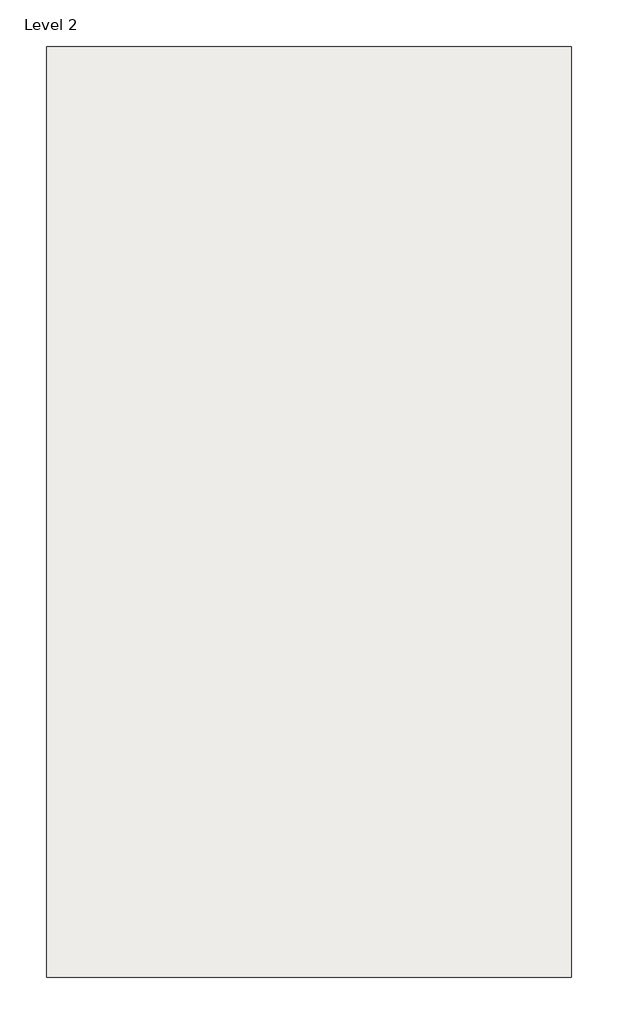
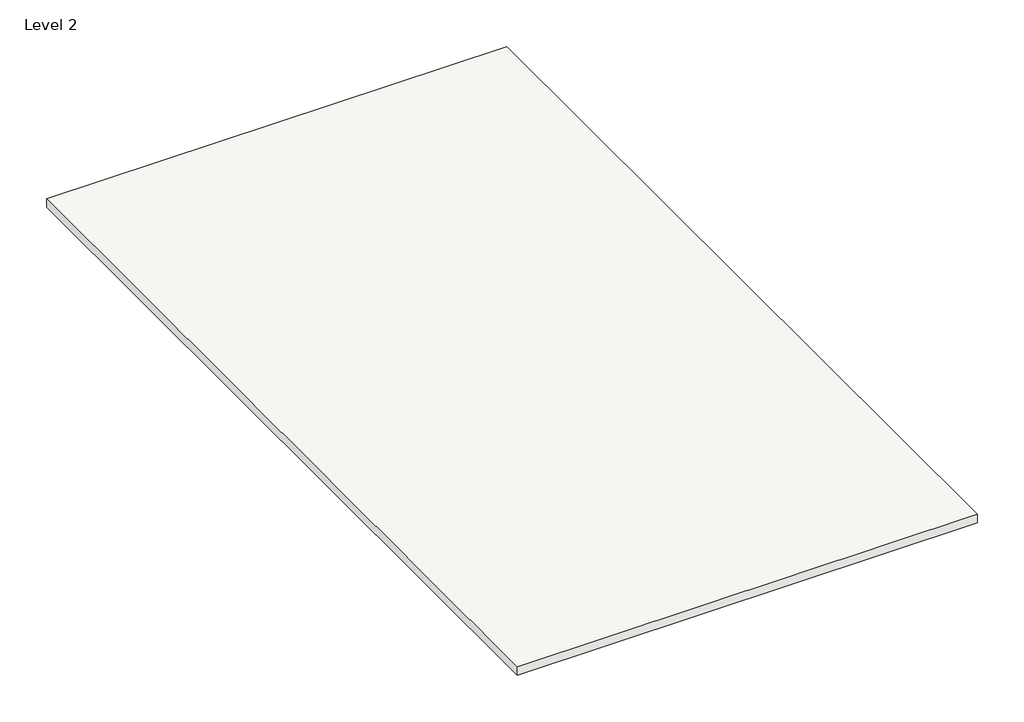
# One storey, incomplete: 1 roof.
"""IFC4 building model written with IfcOpenShell, lengths in millimetres."""

from ifc_helpers import new_model, si_unit, frame, origin, place, context, project, spatial, polyline, outline, extrude, element, save

model = new_model("IFC4")

# Units and contexts
model_context = context("Model", 3, world=origin())
ifc_project = project(units=[si_unit("LENGTHUNIT", "METRE", prefix="MILLI")], contexts=[model_context])

# Site, building, storey
site = spatial("IfcSite", under=ifc_project)
building = spatial("IfcBuilding", under=site)
storey = spatial("IfcBuildingStorey", under=building, Name="Level 2", Elevation=3048.0)

# Roof
placement = place(None, origin())
element("IfcRoof", 1, ObjectType="ROOF 6\"", at=placement, inside=storey, context=model_context, shape_type="SweptSolid", body=[
    extrude(outline(polyline([(-5185.8889285, 7100.4569249), (2675.4110715, 7100.4569249), (2675.4110715, -6831.4430751), (-5185.8889285, -6831.4430751), (-5185.8889285, 7100.4569249)])), frame((0.0, 0.0, 3048.0), z_axis=(0.0, 0.0, 1.0), x_axis=(1.0, 0.0, 0.0)), (0.0, 0.0, 1.0), 152.4),
])

save(model, "model.ifc")

# Revit data of these elements
# Type "ROOF 6\""
#   Assembly Code = "B1020"
#   Layers, outside or top first: 0' - 6" no material (function 1)
# Element 1 (IfcRoof, "ROOF 6\"")
#   built-in parameter 1001705 = 10.5 (stored number, unit not read)
#   built-in parameter 1001710 = 33615
#   Phase Created = New Construction
#   Materials on its faces: "Default Roof", "Door - Panel"
# Materials
#   "Default Roof": colour RGB 88 101 114, transparency 0, Cost = 0
#   "Door - Panel": class "Wood", colour RGB 210 159 95, transparency 0, Cost = 0
